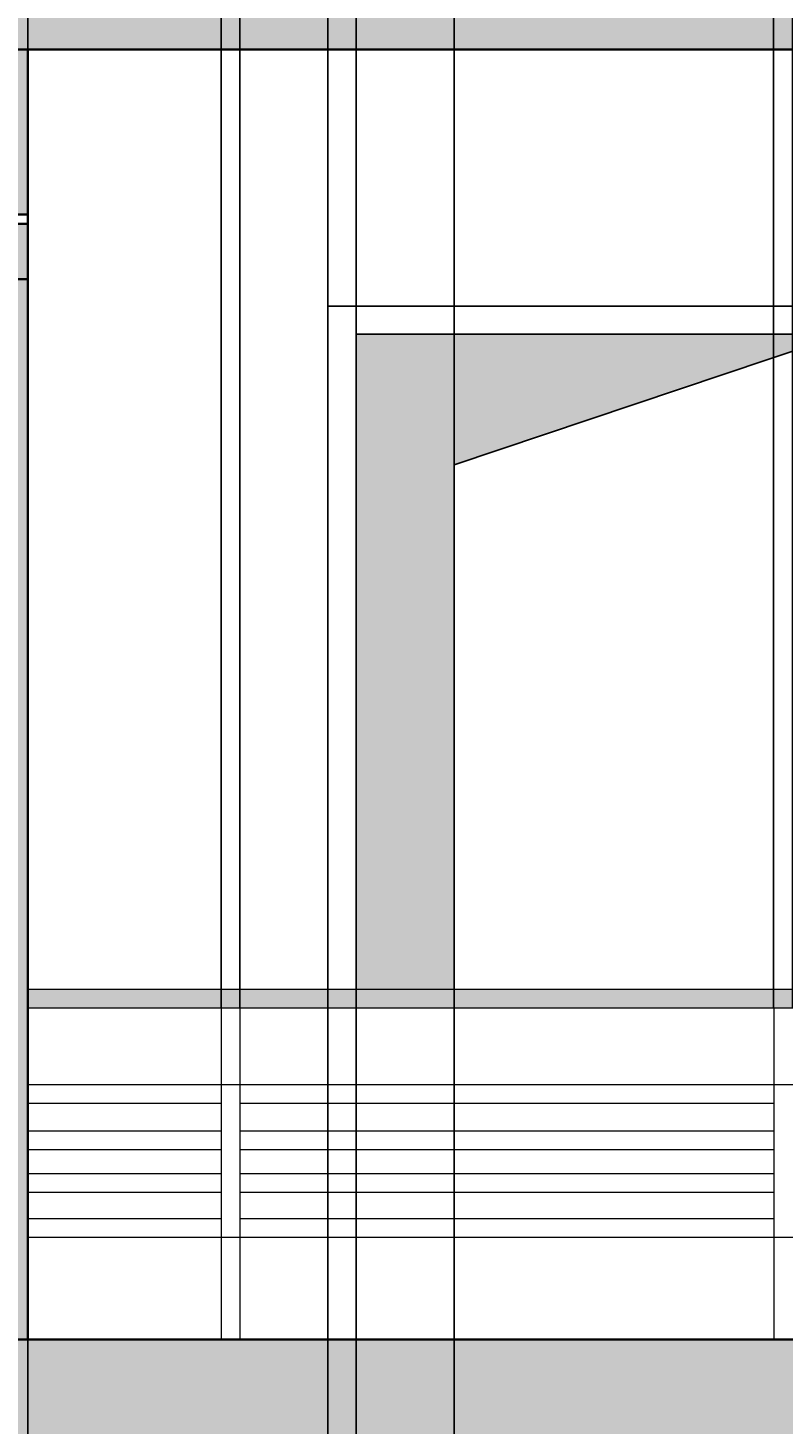
# Model space of a CAD drawing. Units: inches. Extents: x 62 to 566, y 66 to 528.
# Tile 16 of 20: x 284 to 365, y 298 to 447. Entities that reach past the tile are written whole.
import ezdxf

# ---------------------------------------------------------------- set-up
doc = ezdxf.new("R2010")
doc.units = ezdxf.units.IN
doc.header["$MEASUREMENT"] = 0
for name, color, linetype, lineweight in [('A-ANNO-DIMS', 2, 'Continuous', 18), ('A-DOOR', 4, 'Continuous', 25), ('A-ELEV', 7, 'Continuous', 35), ('A-FLOR-HRAL', 6, 'Continuous', 18), ('A-WALL-PATT', 8, 'Continuous', 13)]:
    doc.layers.add(name, color=color, linetype=linetype, lineweight=lineweight)
doc.styles.get("Standard").update_dxf_attribs({"font": 'arial.ttf'})
doc.dimstyles.get("Standard").update_dxf_attribs({"dimtxt": 0.75, "dimasz": 0.18, "dimexe": 0.18, "dimexo": 0.0625, "dimgap": 0.09, "dimtad": 0, "dimtih": 1, "dimtoh": 1, "dimdec": 4, "dimzin": 0, "dimdsep": 46, "dimlunit": 4, "dimtxsty": 'Standard', "dimcen": 0.09, "dimadec": 0, "dimazin": 0, "dimtfac": 1, "dimtdec": 4, "dimtofl": 0, "dimtmove": 0, "dimatfit": 3, "dimfxl": 1, "dimtolj": 1, "dimtzin": 0, "dimarcsym": 0})

# ---------------------------------------------------------------- blocks, each defined once
blk = doc.blocks.new('*D40')
at = {"layer": 'A-ANNO-DIMS', "color": 0, "lineweight": -2, "transparency": 16777216}
for p, q in [((284.2, 445.04), (284.2, 65.94)), ((316.21, 417.64), (316.21, 65.94)), ((284.38, 66.12), (298.92, 66.12)), ((316.03, 66.12), (301.49, 66.12))]:
    blk.add_line(p, q, dxfattribs=at)
at = {"layer": 'A-ANNO-DIMS', "color": 0, "transparency": 16777216}
for points in [[(284.38, 66.15), (284.38, 66.09), (284.2, 66.12)], [(316.03, 66.15), (316.03, 66.09), (316.21, 66.12)]]:
    blk.add_solid(points, dxfattribs=at)
at = {"layer": 'Defpoints', "color": 0, "transparency": 16777216}
for p in [(284.2, 445.11), (316.21, 417.71), (316.21, 66.12)]:
    blk.add_point(p, dxfattribs=at)
at = {"layer": 'A-ANNO-DIMS', "color": 0, "transparency": 16777216, "insert": (300.21, 66.12), "char_height": 0.75, "attachment_point": 5}
blk.add_mtext('\\A1;32.01', dxfattribs=at)
blk = doc.blocks.new('*D41')
at = {"layer": 'A-ANNO-DIMS', "color": 0, "lineweight": -2, "transparency": 16777216}
for p, q in [((316.21, 417.64), (316.21, 65.94)), ((374.14, 417.64), (374.14, 65.94)), ((316.39, 66.12), (343.82, 66.12)), ((373.96, 66.12), (346.53, 66.12))]:
    blk.add_line(p, q, dxfattribs=at)
at = {"layer": 'A-ANNO-DIMS', "color": 0, "transparency": 16777216}
for points in [[(316.39, 66.15), (316.39, 66.09), (316.21, 66.12)], [(373.96, 66.15), (373.96, 66.09), (374.14, 66.12)]]:
    blk.add_solid(points, dxfattribs=at)
at = {"layer": 'Defpoints', "color": 0, "transparency": 16777216}
for p in [(316.21, 417.71), (374.14, 417.71), (374.14, 66.12)]:
    blk.add_point(p, dxfattribs=at)
at = {"layer": 'A-ANNO-DIMS', "color": 0, "transparency": 16777216, "insert": (345.17, 66.12), "char_height": 0.75, "attachment_point": 5}
blk.add_mtext('\\A1;57.93', dxfattribs=at)
blk = doc.blocks.new('*D61')
at = {"layer": 'A-ANNO-DIMS', "color": 0, "lineweight": -2, "transparency": 16777216}
for p, q in [((316.21, 236.72), (316.21, 527.47)), ((319.21, 233.72), (319.21, 527.47)), ((316.39, 527.29), (317.37, 527.29)), ((319.03, 527.29), (318.05, 527.29))]:
    blk.add_line(p, q, dxfattribs=at)
at = {"layer": 'A-ANNO-DIMS', "color": 0, "transparency": 16777216}
for points in [[(316.39, 527.32), (316.39, 527.26), (316.21, 527.29)], [(319.03, 527.32), (319.03, 527.26), (319.21, 527.29)]]:
    blk.add_solid(points, dxfattribs=at)
at = {"layer": 'Defpoints', "color": 0, "transparency": 16777216}
for p in [(319.21, 527.29), (316.21, 236.66), (319.21, 233.66)]:
    blk.add_point(p, dxfattribs=at)
at = {"layer": 'A-ANNO-DIMS', "color": 0, "transparency": 16777216, "insert": (317.71, 527.29), "char_height": 0.75, "attachment_point": 5}
blk.add_mtext('\\A1;3', dxfattribs=at)
blk = doc.blocks.new('*D62')
at = {"layer": 'A-ANNO-DIMS', "color": 0, "lineweight": -2, "transparency": 16777216}
for p, q in [((319.21, 233.72), (319.21, 527.47)), ((329.67, 219.79), (329.67, 527.47)), ((319.39, 527.29), (322.83, 527.29)), ((329.49, 527.29), (326.05, 527.29))]:
    blk.add_line(p, q, dxfattribs=at)
at = {"layer": 'A-ANNO-DIMS', "color": 0, "transparency": 16777216}
for points in [[(319.39, 527.32), (319.39, 527.26), (319.21, 527.29)], [(329.49, 527.32), (329.49, 527.26), (329.67, 527.29)]]:
    blk.add_solid(points, dxfattribs=at)
at = {"layer": 'Defpoints', "color": 0, "transparency": 16777216}
for p in [(329.67, 527.29), (319.21, 233.66), (329.67, 219.73)]:
    blk.add_point(p, dxfattribs=at)
at = {"layer": 'A-ANNO-DIMS', "color": 0, "transparency": 16777216, "insert": (324.44, 527.29), "char_height": 0.75, "attachment_point": 5}
blk.add_mtext('\\A1;10.456', dxfattribs=at)
blk = doc.blocks.new('*D63')
at = {"layer": 'A-ANNO-DIMS', "color": 0, "lineweight": -2, "transparency": 16777216}
for p, q in [((329.67, 219.79), (329.67, 527.47)), ((371.14, 233.72), (371.14, 527.47)), ((329.85, 527.29), (349.03, 527.29)), ((370.96, 527.29), (351.77, 527.29))]:
    blk.add_line(p, q, dxfattribs=at)
at = {"layer": 'A-ANNO-DIMS', "color": 0, "transparency": 16777216}
for points in [[(329.85, 527.32), (329.85, 527.26), (329.67, 527.29)], [(370.96, 527.32), (370.96, 527.26), (371.14, 527.29)]]:
    blk.add_solid(points, dxfattribs=at)
at = {"layer": 'Defpoints', "color": 0, "transparency": 16777216}
for p in [(371.14, 527.29), (371.14, 233.66), (329.67, 219.73)]:
    blk.add_point(p, dxfattribs=at)
at = {"layer": 'A-ANNO-DIMS', "color": 0, "transparency": 16777216, "insert": (350.4, 527.29), "char_height": 0.75, "attachment_point": 5}
blk.add_mtext('\\A1;41.47', dxfattribs=at)
blk = doc.blocks.new('*D74')
at = {"layer": 'A-ANNO-DIMS', "color": 0, "lineweight": -2, "transparency": 16777216}
for p, q in [((284.2, 342.84), (284.2, 527.47)), ((304.82, 342.84), (304.82, 527.47)), ((284.38, 527.29), (292.86, 527.29)), ((304.64, 527.29), (296.16, 527.29))]:
    blk.add_line(p, q, dxfattribs=at)
at = {"layer": 'A-ANNO-DIMS', "color": 0, "transparency": 16777216}
for points in [[(284.38, 527.32), (284.38, 527.26), (284.2, 527.29)], [(304.64, 527.32), (304.64, 527.26), (304.82, 527.29)]]:
    blk.add_solid(points, dxfattribs=at)
at = {"layer": 'Defpoints', "color": 0, "transparency": 16777216}
for p in [(304.82, 527.29), (284.2, 342.78), (304.82, 342.78)]:
    blk.add_point(p, dxfattribs=at)
at = {"layer": 'A-ANNO-DIMS', "color": 0, "transparency": 16777216, "insert": (294.51, 527.29), "char_height": 0.75, "attachment_point": 5}
blk.add_mtext('\\A1;20.614', dxfattribs=at)
blk = doc.blocks.new('*D75')
at = {"layer": 'A-ANNO-DIMS', "color": 0, "lineweight": -2, "transparency": 16777216}
for p, q in [((304.82, 342.84), (304.82, 527.47)), ((306.82, 342.84), (306.82, 527.47)), ((305, 527.29), (305.48, 527.29)), ((306.64, 527.29), (306.15, 527.29))]:
    blk.add_line(p, q, dxfattribs=at)
at = {"layer": 'A-ANNO-DIMS', "color": 0, "transparency": 16777216}
for points in [[(305, 527.32), (305, 527.26), (304.82, 527.29)], [(306.64, 527.32), (306.64, 527.26), (306.82, 527.29)]]:
    blk.add_solid(points, dxfattribs=at)
at = {"layer": 'Defpoints', "color": 0, "transparency": 16777216}
for p in [(306.82, 527.29), (304.82, 342.78), (306.82, 342.78)]:
    blk.add_point(p, dxfattribs=at)
at = {"layer": 'A-ANNO-DIMS', "color": 0, "transparency": 16777216, "insert": (305.82, 527.29), "char_height": 0.75, "attachment_point": 5}
blk.add_mtext('\\A1;2', dxfattribs=at)
blk = doc.blocks.new('*D76')
at = {"layer": 'A-ANNO-DIMS', "color": 0, "lineweight": -2, "transparency": 16777216}
for p, q in [((306.82, 342.84), (306.82, 527.47)), ((363.76, 342.84), (363.76, 527.47)), ((307, 527.29), (333.93, 527.29)), ((363.58, 527.29), (336.65, 527.29))]:
    blk.add_line(p, q, dxfattribs=at)
at = {"layer": 'A-ANNO-DIMS', "color": 0, "transparency": 16777216}
for points in [[(307, 527.32), (307, 527.26), (306.82, 527.29)], [(363.58, 527.32), (363.58, 527.26), (363.76, 527.29)]]:
    blk.add_solid(points, dxfattribs=at)
at = {"layer": 'Defpoints', "color": 0, "transparency": 16777216}
for p in [(363.76, 527.29), (306.82, 342.78), (363.76, 342.78)]:
    blk.add_point(p, dxfattribs=at)
at = {"layer": 'A-ANNO-DIMS', "color": 0, "transparency": 16777216, "insert": (335.29, 527.29), "char_height": 0.75, "attachment_point": 5}
blk.add_mtext('\\A1;56.95', dxfattribs=at)
blk = doc.blocks.new('*D77')
at = {"layer": 'A-ANNO-DIMS', "color": 0, "lineweight": -2, "transparency": 16777216}
for p, q in [((363.76, 342.84), (363.76, 527.47)), ((365.76, 342.84), (365.76, 527.47)), ((363.94, 527.29), (364.43, 527.29)), ((365.58, 527.29), (365.1, 527.29))]:
    blk.add_line(p, q, dxfattribs=at)
at = {"layer": 'A-ANNO-DIMS', "color": 0, "transparency": 16777216}
for points in [[(363.94, 527.32), (363.94, 527.26), (363.76, 527.29)], [(365.58, 527.32), (365.58, 527.26), (365.76, 527.29)]]:
    blk.add_solid(points, dxfattribs=at)
at = {"layer": 'Defpoints', "color": 0, "transparency": 16777216}
for p in [(365.76, 527.29), (363.76, 342.78), (365.76, 342.78)]:
    blk.add_point(p, dxfattribs=at)
at = {"layer": 'A-ANNO-DIMS', "color": 0, "transparency": 16777216, "insert": (364.76, 527.29), "char_height": 0.75, "attachment_point": 5}
blk.add_mtext('\\A1;2', dxfattribs=at)

msp = doc.modelspace()

# ---------------------------------------------------------------- hatches: boundary and pattern name
at = {"layer": 'A-WALL-PATT'}
h = msp.add_hatch(color=256, dxfattribs=at)
h.dxf.hatch_style = 1
h.paths.add_polyline_path([(416.0836, 462.0423), (125.9418, 462.0423), (125.9418, 414.3686), (125.9418, 270.3686), (125.9418, 126.3686), (142.3851, 126.3686), (142.3851, 270.3686), (142.3851, 414.3686), (142.3851, 445.1064), (284.2021, 445.1064), (416.0836, 445.1064)])
h.paths.add_polyline_path([(435.3945, 503.0423), (426.3652, 503.0423), (120.4058, 503.0423), (120.4058, 501.0423), (125.9418, 501.0423), (416.0836, 501.0423), (426.3652, 501.0423), (430.6938, 501.0423), (435.3945, 501.0423)])
h.paths.add_polyline_path([(439.6878, 352.4848), (392.4793, 352.4848), (392.4793, 307.4128), (217.2752, 307.4128), (217.2752, 295.4098), (217.2752, 271.4128), (272.0586, 271.4128), (439.6878, 271.4128)])
h.paths.add_polyline_path([(248.0143, 297.1682), (255.6783, 297.1682), (255.6783, 280.0423), (248.0143, 280.0423)], flags=16)
h.paths.add_polyline_path([(235.4641, 280.0423), (227.8001, 280.0423), (227.8001, 297.1682), (235.4641, 297.1682)], flags=16)
h.paths.add_polyline_path([(270.4427, 297.1682), (278.1067, 297.1682), (278.1067, 280.0423), (270.4427, 280.0423)], flags=16)
h.paths.add_polyline_path([(296.3755, 297.1682), (304.0395, 297.1682), (304.0395, 280.0423), (296.3755, 280.0423)], flags=16)
h.paths.add_polyline_path([(319.2543, 297.1682), (326.9183, 297.1682), (326.9183, 280.0423), (319.2543, 280.0423)], flags=16)
h.paths.add_polyline_path([(341.2622, 297.1682), (348.9262, 297.1682), (348.9262, 280.0423), (341.2622, 280.0423)], flags=16)
h.paths.add_polyline_path([(389.2857, 298.3985), (433.8102, 298.3985), (433.8102, 294.9497), (389.2857, 294.9497)], flags=16)
h.paths.add_polyline_path([(389.2857, 291.6038), (433.8102, 291.6038), (433.8102, 288.155), (389.2857, 288.155)], flags=16)
h.paths.add_polyline_path([(389.2857, 284.9607), (433.8102, 284.9607), (433.8102, 281.5119), (389.2857, 281.5119)], flags=16)
h.paths.add_polyline_path([(403.5849, 311.4736), (403.5849, 317.4388), (433.1636, 317.4388), (433.1636, 311.4736)], flags=16)
h.paths.add_polyline_path([(403.5849, 323.1329), (403.5849, 329.0982), (433.1636, 329.0982), (433.1636, 323.1329)], flags=16)
h.paths.add_polyline_path([(403.5849, 334.5211), (403.5849, 340.4863), (433.1636, 340.4863), (433.1636, 334.5211)], flags=16)
h.paths.add_polyline_path([(272.0586, 160.3545), (217.2752, 160.3545), (217.2752, 129.0504), (217.2752, 126.3686), (272.0586, 126.3686)], flags=17)
h.paths.add_polyline_path([(220.5897, 149.5749), (220.5897, 152.296), (267.7931, 152.296), (267.7931, 149.5749)], flags=16)
h.paths.add_polyline_path([(267.7931, 146.6724), (267.7931, 143.9513), (220.5897, 143.9513), (220.5897, 146.6724)], flags=16)
h.paths.add_polyline_path([(220.5897, 155.3799), (220.5897, 158.101), (267.7931, 158.101), (267.7931, 155.3799)], flags=16)
h.paths.add_polyline_path([(267.7931, 140.686), (267.7931, 137.9649), (220.5897, 137.9649), (220.5897, 140.686)], flags=16)
h.paths.add_polyline_path([(267.7931, 135.516), (267.7931, 132.7949), (220.5897, 132.7949), (220.5897, 135.516)], flags=16)
h = msp.add_hatch(color=256, dxfattribs=at)
h.dxf.hatch_style = 1
h.paths.add_polyline_path([(416.0836, 501.0423), (282.3509, 501.0423), (282.3509, 465.0423), (416.0836, 465.0423)])
h.paths.add_polyline_path([(284.2021, 420.597), (272.0586, 420.597), (272.0586, 309.5388), (272.0586, 307.4128), (284.2021, 307.4128)], flags=17)
h.paths.add_polyline_path([(284.2021, 445.1064), (142.3851, 445.1064), (142.3851, 414.3686), (142.3851, 270.3686), (142.3851, 126.3686), (163.6548, 126.3686), (163.6548, 270.5016), (163.6548, 414.5016), (163.6548, 427.4752), (284.2021, 427.4752)])
h.paths.add_polyline_path([(235.4641, 297.1682), (227.8001, 297.1682), (227.8001, 280.0423), (235.4641, 280.0423)], flags=17)
h.paths.add_polyline_path([(255.6783, 297.1682), (248.0143, 297.1682), (248.0143, 280.0423), (255.6783, 280.0423)], flags=17)
h.paths.add_polyline_path([(278.1067, 297.1682), (270.4427, 297.1682), (270.4427, 280.0423), (278.1067, 280.0423)], flags=17)
h.paths.add_polyline_path([(304.0395, 297.1682), (296.3755, 297.1682), (296.3755, 280.0423), (304.0395, 280.0423)])
h.paths.add_polyline_path([(326.9183, 297.1682), (319.2543, 297.1682), (319.2543, 280.0423), (326.9183, 280.0423)])
h.paths.add_polyline_path([(348.9262, 297.1682), (341.2622, 297.1682), (341.2622, 280.0423), (348.9262, 280.0423)])
h.paths.add_polyline_path([(433.8102, 284.9607), (389.2857, 284.9607), (389.2857, 281.5119), (433.8102, 281.5119)])
h.paths.add_polyline_path([(433.8102, 291.6038), (389.2857, 291.6038), (389.2857, 288.155), (433.8102, 288.155)])
h.paths.add_polyline_path([(433.8102, 298.3985), (389.2857, 298.3985), (389.2857, 294.9497), (433.8102, 294.9497)])
h.paths.add_polyline_path([(433.1636, 317.4388), (403.5849, 317.4388), (403.5849, 311.4736), (433.1636, 311.4736)])
h.paths.add_polyline_path([(433.1636, 329.0982), (403.5849, 329.0982), (403.5849, 323.1329), (433.1636, 323.1329)])
h.paths.add_polyline_path([(433.1636, 340.4863), (403.5849, 340.4863), (403.5849, 334.5211), (433.1636, 334.5211)])
h.paths.add_polyline_path([(284.2021, 271.4128), (272.0586, 271.4128), (272.0586, 160.3545), (272.0586, 126.3686), (284.2021, 126.3686)])
h.paths.add_polyline_path([(267.7931, 158.101), (220.5897, 158.101), (220.5897, 155.3799), (267.7931, 155.3799)], flags=17)
h.paths.add_polyline_path([(267.7931, 152.296), (220.5897, 152.296), (220.5897, 149.5749), (267.7931, 149.5749)], flags=17)
h.paths.add_polyline_path([(267.7931, 146.6724), (220.5897, 146.6724), (220.5897, 143.9513), (267.7931, 143.9513)], flags=17)
h.paths.add_polyline_path([(267.7931, 140.686), (220.5897, 140.686), (220.5897, 137.9649), (267.7931, 137.9649)], flags=17)
h.paths.add_polyline_path([(267.7931, 135.516), (220.5897, 135.516), (220.5897, 132.7949), (267.7931, 132.7949)], flags=17)
h.paths.add_polyline_path([(148.2354, 493.4274), (140.5713, 493.4274), (140.5713, 476.3015), (148.2354, 476.3015)])
h.paths.add_polyline_path([(163.2545, 493.4274), (155.5905, 493.4274), (155.5905, 476.3015), (163.2545, 476.3015)])
h.paths.add_polyline_path([(177.9243, 493.7764), (170.2603, 493.7764), (170.2603, 476.6506), (177.9243, 476.6506)])
h.paths.add_polyline_path([(193.9913, 493.7764), (186.3273, 493.7764), (186.3273, 476.6506), (193.9913, 476.6506)])
h.paths.add_polyline_path([(209.709, 493.7764), (202.045, 493.7764), (202.045, 476.6506), (209.709, 476.6506)])
h = msp.add_hatch(color=256, dxfattribs=at)
h.dxf.hatch_style = 1
h.paths.add_polyline_path([(430.6938, 462.0423), (416.0836, 462.0423), (416.0836, 445.1064), (430.6938, 445.1064)])
h.paths.add_polyline_path([(169.0431, 420.597), (284.2021, 420.597), (284.2021, 426.4752), (164.6548, 426.4752), (164.6548, 414.5016), (164.6548, 126.3686), (169.0431, 126.3686)])
h = msp.add_hatch(color=256, dxfattribs=at)
h.dxf.hatch_style = 1
h.paths.add_polyline_path([(371.1373, 233.6618), (319.2101, 233.6618), (319.2101, 129.3686), (329.6665, 129.3686), (329.6665, 219.7304)])
h.paths.add_polyline_path([(371.1373, 414.7059), (319.2101, 414.7059), (319.2101, 344.7821), (329.6665, 344.7821), (329.6665, 400.7745)])
h.paths.add_polyline_path([(392.4793, 344.7821), (284.2021, 344.7821), (284.2021, 342.7821), (392.4793, 342.7821)])

# ---------------------------------------------------------------- linework, layer by layer
at = {"layer": 'A-DOOR'}
for p, q in [((371.1373, 414.7059), (329.6665, 400.7745)), ((329.6665, 400.7745), (329.6665, 344.7821))]:
    msp.add_line(p, q, dxfattribs=at)
for points in [[(316.2101, 344.7821), (316.2101, 417.7059), (374.1373, 417.7059), (374.1373, 344.7821)], [(319.2101, 344.7821), (319.2101, 414.7059), (371.1373, 414.7059), (371.1373, 344.7821)], [(374.1373, 307.4128), (316.2101, 307.4128)]]:
    msp.add_lwpolyline(points, dxfattribs=at)
at = {"layer": 'A-ELEV'}
for p, q in [((142.3851, 445.1064), (284.2021, 445.1064)), ((284.2021, 445.1064), (284.2021, 427.4752)), ((284.2021, 445.1064), (416.0836, 445.1064)), ((284.2021, 420.597), (284.2021, 307.4128)), ((217.2752, 307.4128), (392.4793, 307.4128))]:
    msp.add_line(p, q, dxfattribs=at)
for points in [[(163.6548, 126.3686), (163.6548, 414.5016), (163.6548, 427.4752), (284.2021, 427.4752)], [(164.6548, 126.3686), (164.6548, 414.5016), (164.6548, 426.4752), (284.2021, 426.4752)], [(169.0431, 420.597), (284.2021, 420.597), (284.2021, 427.4752)]]:
    msp.add_lwpolyline(points, dxfattribs=at)
at = {"layer": 'A-FLOR-HRAL'}
for p, q in [((392.4793, 344.7821), (284.2021, 344.7821)), ((392.4793, 342.7821), (284.2021, 342.7821)), ((304.8163, 342.7821), (304.8163, 307.4128)), ((306.8163, 342.7821), (306.8163, 307.4128)), ((363.764, 342.7821), (363.764, 307.4128)), ((392.4793, 334.6119), (284.2021, 334.6119)), ((304.8163, 332.6119), (284.2021, 332.6119)), ((363.764, 332.6119), (306.8163, 332.6119)), ((304.8163, 329.6741), (284.2021, 329.6741)), ((363.764, 329.6741), (306.8163, 329.6741)), ((304.8163, 327.6741), (284.2021, 327.6741)), ((363.764, 327.6741), (306.8163, 327.6741)), ((304.8163, 325.1162), (284.2021, 325.1162)), ((363.764, 325.1162), (306.8163, 325.1162)), ((304.8163, 323.1162), (284.2021, 323.1162)), ((363.764, 323.1162), (306.8163, 323.1162)), ((304.8163, 320.3051), (284.2021, 320.3051)), ((363.764, 320.3051), (306.8163, 320.3051)), ((392.4793, 318.3051), (284.2021, 318.3051))]:
    msp.add_line(p, q, dxfattribs=at)

# ---------------------------------------------------------------- dimensions: what is measured, and where the dimension line sits
at = {"layer": 'A-ANNO-DIMS'}
for base, p1, p2, override, picture, middle in [((304.8163, 527.2923), (284.2021, 342.7821), (304.8163, 342.7821), {"dimdec": 3, "dimlfac": 1, "dimrnd": 0, "dimzin": 0, "dimdsep": 46, "dimlunit": 2}, '*D74', (294.5092, 527.2923)), ((306.8163, 527.2923), (304.8163, 342.7821), (306.8163, 342.7821), {"dimdec": 0, "dimlfac": 1, "dimrnd": 0, "dimzin": 0, "dimdsep": 46, "dimlunit": 2}, '*D75', (305.8163, 527.2923)), ((363.764, 527.2923), (306.8163, 342.7821), (363.764, 342.7821), {"dimdec": 2, "dimlfac": 1, "dimrnd": 0, "dimzin": 0, "dimdsep": 46, "dimlunit": 2}, '*D76', (335.2902, 527.2923)), ((319.2101, 527.2923), (316.2101, 236.6618), (319.2101, 233.6618), {"dimdec": 0, "dimlfac": 1, "dimrnd": 0, "dimzin": 0, "dimdsep": 46, "dimlunit": 2}, '*D61', (317.7101, 527.2923)), ((329.6665, 527.2923), (319.2101, 233.6618), (329.6665, 219.7304), {"dimdec": 3, "dimlfac": 1, "dimrnd": 0, "dimzin": 0, "dimdsep": 46, "dimlunit": 2}, '*D62', (324.4383, 527.2923)), ((371.1373, 527.2923), (329.6665, 219.7304), (371.1373, 233.6618), {"dimdec": 2, "dimlfac": 1, "dimrnd": 0, "dimzin": 0, "dimdsep": 46, "dimlunit": 2}, '*D63', (350.4019, 527.2923)), ((365.764, 527.2923), (363.764, 342.7821), (365.764, 342.7821), {"dimdec": 0, "dimlfac": 1, "dimrnd": 0, "dimzin": 0, "dimdsep": 46, "dimlunit": 2}, '*D77', (364.764, 527.2923)), ((316.2101, 66.1186), (284.2021, 445.1064), (316.2101, 417.7059), {"dimdec": 2, "dimlfac": 1, "dimrnd": 0, "dimzin": 0, "dimdsep": 46, "dimlunit": 2}, '*D40', (300.2061, 66.1186)), ((374.1373, 66.1186), (316.2101, 417.7059), (374.1373, 417.7059), {"dimdec": 2, "dimlfac": 1, "dimrnd": 0, "dimzin": 0, "dimdsep": 46, "dimlunit": 2}, '*D41', (345.1737, 66.1186))]:
    dim = msp.add_linear_dim(base=base, p1=p1, p2=p2, dimstyle='Standard', override=override, dxfattribs=at)
    dim.commit()
    dim.dimension.update_dxf_attribs({"geometry": picture, "text_midpoint": middle})

doc.saveas('drawing.dxf')
